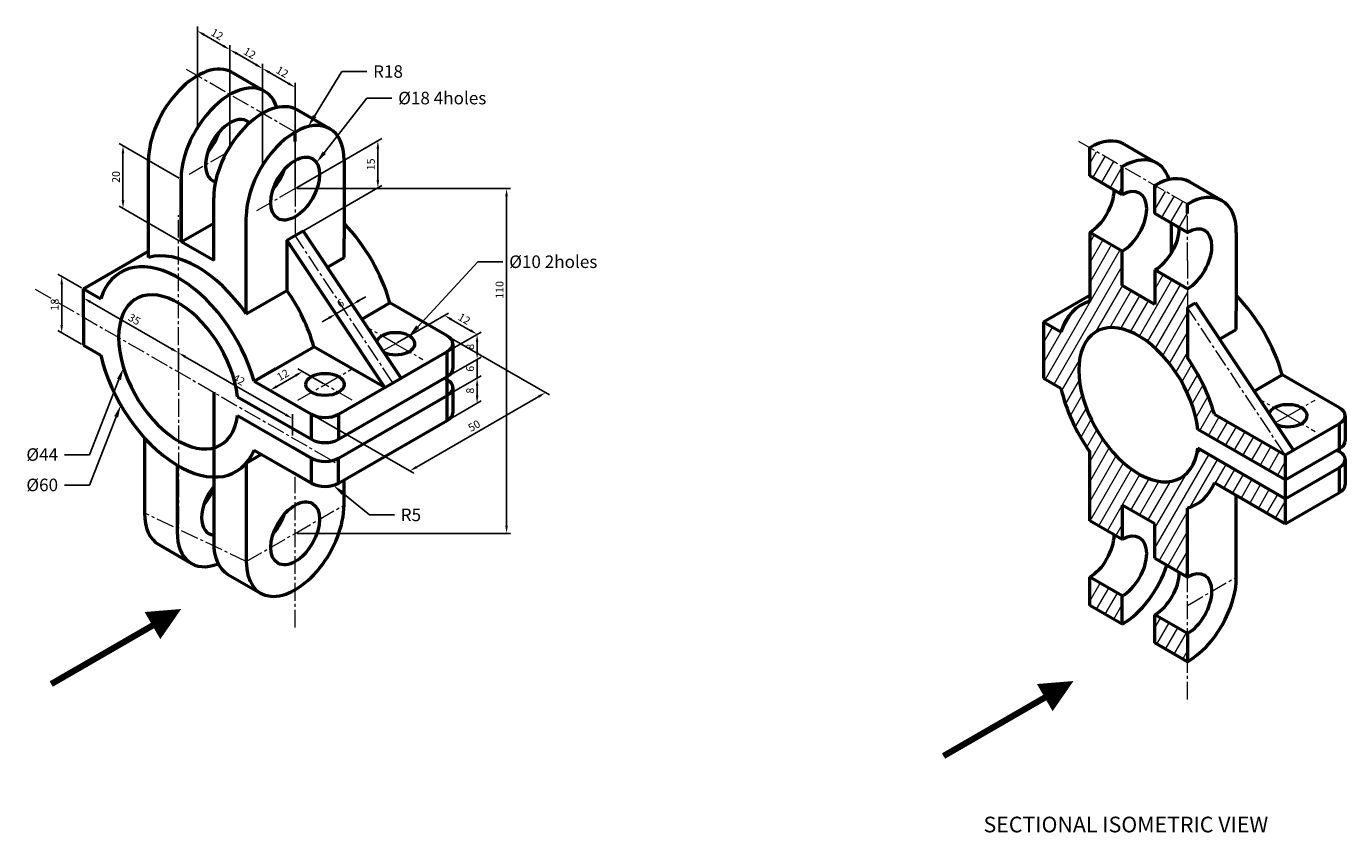
# Model space of a CAD drawing. Units: millimetres. Extents: x 2364 to 2785, y 1000 to 1694.
# Tile 2 of 2: x 2364 to 2785, y 1437 to 1694. Entities that reach past the tile are written whole.
import ezdxf
from ezdxf import colors
from ezdxf.entities.mleader import LeaderData, LeaderLine
from ezdxf.math import Vec2, Vec3

# ---------------------------------------------------------------- set-up
doc = ezdxf.new("R2010")
doc.units = ezdxf.units.MM
doc.linetypes.add('CENTER2', pattern=[28.575, 19.05, -3.175, 3.175, -3.175])
for name, color, linetype, lineweight in [('M-CNTR', 1, 'CENTER2', 18), ('M-DIMS', 2, 'Continuous', 25), ('M-HATC', 8, 'Continuous', 18), ('M-OUTL', 7, 'Continuous', 50), ('M-SYMB', 7, 'Continuous', 18), ('M-TEXT', 3, 'Continuous', 25)]:
    doc.layers.add(name, color=color, linetype=linetype, lineweight=lineweight)
doc.styles.get("Standard").update_dxf_attribs({"font": 'arial.ttf'})
doc.dimstyles.new('ISO-25', dxfattribs={"dimtxt": 2.5, "dimasz": 2.5, "dimexe": 1.25, "dimexo": 0.625, "dimtad": 1, "dimtxsty": 'Standard', "dimcen": 2.5, "dimadec": 0, "dimazin": 0, "dimtfac": 1, "dimtmove": 0, "dimatfit": 3, "dimfxl": 1, "dimarcsym": 0})
pattern_1 = [(60, (-235.2593, 567.1468), (-2.7496307, 1.5875), [])]

# ---------------------------------------------------------------- blocks, each defined once
blk = doc.blocks.new('*D1')
at = {"layer": 'Defpoints', "color": 0, "transparency": 16777216}
for p in [(2439.77, 1680.8), (2439.77, 1648.49), (2450.16, 1642.49)]:
    blk.add_point(p, dxfattribs=at)
at = {"layer": 'M-DIMS', "color": 0, "lineweight": -2, "transparency": 16777216}
for p, q in [((2439.77, 1649.21), (2439.77, 1682.25)), ((2448, 1676.05), (2441.94, 1679.55)), ((2450.16, 1643.21), (2450.16, 1676.25))]:
    blk.add_line(p, q, dxfattribs=at)
at = {"layer": 'M-DIMS', "color": 0, "transparency": 16777216}
for points in [[(2442.15, 1679.91), (2441.73, 1679.19), (2439.77, 1680.8)], [(2448.21, 1676.41), (2447.79, 1675.69), (2450.16, 1674.8)]]:
    blk.add_solid(points, dxfattribs=at)
at = {"layer": 'M-DIMS', "color": 0, "transparency": 16777216, "insert": (2445.91, 1679.43), "char_height": 2.5, "attachment_point": 5, "rotation": 330}
blk.add_mtext('12', dxfattribs=at)
blk = doc.blocks.new('*D2')
at = {"layer": 'Defpoints', "color": 0, "transparency": 16777216}
for p in [(2429.38, 1686.8), (2429.38, 1654.49), (2439.77, 1648.49)]:
    blk.add_point(p, dxfattribs=at)
at = {"layer": 'M-DIMS', "color": 0, "lineweight": -2, "transparency": 16777216}
for p, q in [((2429.38, 1655.21), (2429.38, 1688.25)), ((2437.61, 1682.05), (2431.55, 1685.55)), ((2439.77, 1649.21), (2439.77, 1682.25))]:
    blk.add_line(p, q, dxfattribs=at)
at = {"layer": 'M-DIMS', "color": 0, "transparency": 16777216}
for points in [[(2431.75, 1685.91), (2431.34, 1685.19), (2429.38, 1686.8)], [(2437.82, 1682.41), (2437.4, 1681.69), (2439.77, 1680.8)]]:
    blk.add_solid(points, dxfattribs=at)
at = {"layer": 'M-DIMS', "color": 0, "transparency": 16777216, "insert": (2435.52, 1685.43), "char_height": 2.5, "attachment_point": 5, "rotation": 330}
blk.add_mtext('12', dxfattribs=at)
blk = doc.blocks.new('*D3')
at = {"layer": 'Defpoints', "color": 0, "transparency": 16777216}
for p in [(2418.99, 1692.8), (2418.99, 1660.49), (2429.38, 1654.49)]:
    blk.add_point(p, dxfattribs=at)
at = {"layer": 'M-DIMS', "color": 0, "lineweight": -2, "transparency": 16777216}
for p, q in [((2418.99, 1661.21), (2418.99, 1694.25)), ((2427.22, 1688.05), (2421.15, 1691.55)), ((2429.38, 1655.21), (2429.38, 1688.25))]:
    blk.add_line(p, q, dxfattribs=at)
at = {"layer": 'M-DIMS', "color": 0, "transparency": 16777216}
for points in [[(2421.36, 1691.91), (2420.94, 1691.19), (2418.99, 1692.8)], [(2427.42, 1688.41), (2427.01, 1687.69), (2429.38, 1686.8)]]:
    blk.add_solid(points, dxfattribs=at)
at = {"layer": 'M-DIMS', "color": 0, "transparency": 16777216, "insert": (2425.12, 1691.43), "char_height": 2.5, "attachment_point": 5, "rotation": 330}
blk.add_mtext('12', dxfattribs=at)
blk = doc.blocks.new('*D4')
at = {"layer": 'Defpoints', "color": 0, "transparency": 16777216}
for p in [(2413.79, 1645.49), (2395.26, 1636.19), (2413.79, 1625.49)]:
    blk.add_point(p, dxfattribs=at)
at = {"layer": 'M-DIMS', "color": 0, "lineweight": -2, "transparency": 16777216}
for p, q in [((2413.17, 1645.85), (2394.01, 1656.91)), ((2395.26, 1653.69), (2395.26, 1638.69)), ((2413.17, 1625.85), (2394.01, 1636.91))]:
    blk.add_line(p, q, dxfattribs=at)
at = {"layer": 'M-DIMS', "color": 0, "transparency": 16777216}
for points in [[(2394.84, 1653.69), (2395.68, 1653.69), (2395.26, 1656.19)], [(2394.84, 1638.69), (2395.68, 1638.69), (2395.26, 1636.19)]]:
    blk.add_solid(points, dxfattribs=at)
at = {"layer": 'M-DIMS', "color": 0, "transparency": 16777216, "insert": (2393.36, 1646.19), "char_height": 2.5, "attachment_point": 5, "rotation": 90}
blk.add_mtext('20', dxfattribs=at)
blk = doc.blocks.new('*D5')
at = {"layer": 'Defpoints', "color": 0, "transparency": 16777216}
for p in [(2450.16, 1642.49), (2476.54, 1642.72), (2450.16, 1627.49)]:
    blk.add_point(p, dxfattribs=at)
at = {"layer": 'M-DIMS', "color": 0, "lineweight": -2, "transparency": 16777216}
for p, q in [((2450.79, 1642.85), (2477.79, 1658.44)), ((2476.54, 1655.22), (2476.54, 1645.22)), ((2450.79, 1627.85), (2477.79, 1643.44))]:
    blk.add_line(p, q, dxfattribs=at)
at = {"layer": 'M-DIMS', "color": 0, "transparency": 16777216}
for points in [[(2476.13, 1655.22), (2476.96, 1655.22), (2476.54, 1657.72)], [(2476.13, 1645.22), (2476.96, 1645.22), (2476.54, 1642.72)]]:
    blk.add_solid(points, dxfattribs=at)
at = {"layer": 'M-DIMS', "color": 0, "transparency": 16777216, "insert": (2474.64, 1650.22), "char_height": 2.5, "attachment_point": 5, "rotation": 90}
blk.add_mtext('15', dxfattribs=at)
blk = doc.blocks.new('*D6')
at = {"layer": 'Defpoints', "color": 0, "transparency": 16777216}
for p in [(2442.14, 1578.13), (2459.69, 1579.99), (2449.3, 1573.99)]:
    blk.add_point(p, dxfattribs=at)
at = {"layer": 'M-DIMS', "color": 0, "lineweight": -2, "transparency": 16777216}
for p, q in [((2450.37, 1582.88), (2444.31, 1579.38)), ((2459.07, 1580.35), (2451.28, 1584.85)), ((2448.67, 1574.35), (2440.89, 1578.85))]:
    blk.add_line(p, q, dxfattribs=at)
at = {"layer": 'M-DIMS', "color": 0, "transparency": 16777216}
for points in [[(2450.16, 1583.24), (2450.58, 1582.51), (2452.53, 1584.13)], [(2444.1, 1579.74), (2444.51, 1579.01), (2442.14, 1578.13)]]:
    blk.add_solid(points, dxfattribs=at)
at = {"layer": 'M-DIMS', "color": 0, "transparency": 16777216, "insert": (2446.4, 1582.75), "char_height": 2.5, "attachment_point": 5, "rotation": 30}
blk.add_mtext('12', dxfattribs=at)
blk = doc.blocks.new('*D7')
at = {"layer": 'Defpoints', "color": 0, "transparency": 16777216}
for p in [(2508.2, 1596), (2482.21, 1592.99), (2492.6, 1586.99)]:
    blk.add_point(p, dxfattribs=at)
at = {"layer": 'M-DIMS', "color": 0, "lineweight": -2, "transparency": 16777216}
for p, q in [((2482.83, 1593.35), (2499.06, 1602.72)), ((2499.98, 1600.75), (2506.04, 1597.25)), ((2493.22, 1587.35), (2509.45, 1596.72))]:
    blk.add_line(p, q, dxfattribs=at)
at = {"layer": 'M-DIMS', "color": 0, "transparency": 16777216}
for points in [[(2500.19, 1601.11), (2499.77, 1600.39), (2497.81, 1602)], [(2506.25, 1597.61), (2505.83, 1596.89), (2508.2, 1596)]]:
    blk.add_solid(points, dxfattribs=at)
at = {"layer": 'M-DIMS', "color": 0, "transparency": 16777216, "insert": (2503.95, 1600.63), "char_height": 2.5, "attachment_point": 5, "rotation": 330}
blk.add_mtext('12', dxfattribs=at)
blk = doc.blocks.new('*D8')
at = {"layer": 'Defpoints', "color": 0, "transparency": 16777216}
for p in [(2498.66, 1576.49), (2508.2, 1574), (2498.66, 1568.49)]:
    blk.add_point(p, dxfattribs=at)
at = {"layer": 'M-DIMS', "color": 0, "lineweight": -2, "transparency": 16777216}
for p, q in [((2499.29, 1576.85), (2509.45, 1582.72)), ((2508.2, 1579.5), (2508.2, 1576.5)), ((2499.29, 1568.85), (2509.45, 1574.72))]:
    blk.add_line(p, q, dxfattribs=at)
at = {"layer": 'M-DIMS', "color": 0, "transparency": 16777216}
for points in [[(2507.79, 1579.5), (2508.62, 1579.5), (2508.2, 1582)], [(2507.79, 1576.5), (2508.62, 1576.5), (2508.2, 1574)]]:
    blk.add_solid(points, dxfattribs=at)
at = {"layer": 'M-DIMS', "color": 0, "transparency": 16777216, "insert": (2506.3, 1578), "char_height": 2.5, "attachment_point": 5, "rotation": 90}
blk.add_mtext('8', dxfattribs=at)
blk = doc.blocks.new('*D9')
at = {"layer": 'Defpoints', "color": 0, "transparency": 16777216}
for p in [(2508.2, 1588), (2498.66, 1582.49), (2498.66, 1576.49)]:
    blk.add_point(p, dxfattribs=at)
at = {"layer": 'M-DIMS', "color": 0, "lineweight": -2, "transparency": 16777216}
for p, q in [((2508.2, 1590.5), (2508.2, 1593)), ((2499.29, 1582.85), (2509.45, 1588.72)), ((2508.2, 1582), (2508.2, 1588)), ((2499.29, 1576.85), (2509.45, 1582.72)), ((2508.2, 1579.5), (2508.2, 1577))]:
    blk.add_line(p, q, dxfattribs=at)
at = {"layer": 'M-DIMS', "color": 0, "transparency": 16777216}
for points in [[(2507.79, 1590.5), (2508.62, 1590.5), (2508.2, 1588)], [(2507.79, 1579.5), (2508.62, 1579.5), (2508.2, 1582)]]:
    blk.add_solid(points, dxfattribs=at)
at = {"layer": 'M-DIMS', "color": 0, "transparency": 16777216, "insert": (2506.3, 1585), "char_height": 2.5, "attachment_point": 5, "rotation": 90}
blk.add_mtext('6', dxfattribs=at)
blk = doc.blocks.new('*D10')
at = {"layer": 'Defpoints', "color": 0, "transparency": 16777216}
for p in [(2508.2, 1596), (2498.66, 1590.49), (2498.66, 1582.49)]:
    blk.add_point(p, dxfattribs=at)
at = {"layer": 'M-DIMS', "color": 0, "lineweight": -2, "transparency": 16777216}
for p, q in [((2499.29, 1590.85), (2509.45, 1596.72)), ((2508.2, 1590.5), (2508.2, 1593.5)), ((2499.29, 1582.85), (2509.45, 1588.72))]:
    blk.add_line(p, q, dxfattribs=at)
at = {"layer": 'M-DIMS', "color": 0, "transparency": 16777216}
for points in [[(2507.79, 1593.5), (2508.62, 1593.5), (2508.2, 1596)], [(2507.79, 1590.5), (2508.62, 1590.5), (2508.2, 1588)]]:
    blk.add_solid(points, dxfattribs=at)
at = {"layer": 'M-DIMS', "color": 0, "transparency": 16777216, "insert": (2506.3, 1592), "char_height": 2.5, "attachment_point": 5, "rotation": 90}
blk.add_mtext('8', dxfattribs=at)
blk = doc.blocks.new('*D11')
at = {"layer": 'Defpoints', "color": 0, "transparency": 16777216}
for p in [(2450.16, 1642.49), (2517.59, 1642.49), (2450.16, 1532.49)]:
    blk.add_point(p, dxfattribs=at)
at = {"layer": 'M-DIMS', "color": 0, "lineweight": -2, "transparency": 16777216}
for p, q in [((2450.79, 1642.49), (2518.84, 1642.49)), ((2517.59, 1534.99), (2517.59, 1639.99)), ((2450.79, 1532.49), (2518.84, 1532.49))]:
    blk.add_line(p, q, dxfattribs=at)
at = {"layer": 'M-DIMS', "color": 0, "transparency": 16777216}
for points in [[(2517.17, 1639.99), (2518, 1639.99), (2517.59, 1642.49)], [(2517.17, 1534.99), (2518, 1534.99), (2517.59, 1532.49)]]:
    blk.add_solid(points, dxfattribs=at)
at = {"layer": 'M-DIMS', "color": 0, "transparency": 16777216, "insert": (2515.68, 1610.16), "char_height": 2.5, "attachment_point": 5, "rotation": 90}
blk.add_mtext('110', dxfattribs=at)
blk = doc.blocks.new('*D12')
at = {"layer": 'Defpoints', "color": 0, "transparency": 16777216}
for p in [(2498.66, 1595.49), (2530.02, 1577.39), (2455.36, 1570.49)]:
    blk.add_point(p, dxfattribs=at)
at = {"layer": 'M-DIMS', "color": 0, "lineweight": -2, "transparency": 16777216}
for p, q in [((2499.29, 1595.13), (2531.27, 1576.67)), ((2488.88, 1553.64), (2527.85, 1576.14)), ((2455.99, 1570.13), (2487.97, 1551.67))]:
    blk.add_line(p, q, dxfattribs=at)
at = {"layer": 'M-DIMS', "color": 0, "transparency": 16777216}
for points in [[(2527.64, 1576.5), (2528.06, 1575.78), (2530.02, 1577.39)], [(2488.67, 1554), (2489.09, 1553.28), (2486.72, 1552.39)]]:
    blk.add_solid(points, dxfattribs=at)
at = {"layer": 'M-DIMS', "color": 0, "transparency": 16777216, "insert": (2507.42, 1566.54), "char_height": 2.5, "attachment_point": 5, "rotation": 30}
blk.add_mtext('50', dxfattribs=at)
blk = doc.blocks.new('*D13')
at = {"layer": 'Defpoints', "color": 0, "transparency": 16777216}
for p in [(2468.35, 1605.49), (2468.35, 1605.49), (2463.16, 1602.49)]:
    blk.add_point(p, dxfattribs=at)
at = {"layer": 'M-DIMS', "color": 0, "lineweight": -2, "transparency": 16777216}
for p, q in [((2470.52, 1606.74), (2472.68, 1607.99)), ((2462.84, 1603.03), (2462.53, 1603.58)), ((2463.16, 1602.49), (2468.35, 1605.49)), ((2468.04, 1606.03), (2467.73, 1606.58)), ((2460.99, 1601.24), (2458.82, 1599.99))]:
    blk.add_line(p, q, dxfattribs=at)
at = {"layer": 'M-DIMS', "color": 0, "transparency": 16777216}
for points in [[(2470.31, 1607.1), (2470.72, 1606.38), (2468.35, 1605.49)], [(2460.78, 1601.6), (2461.2, 1600.88), (2463.16, 1602.49)]]:
    blk.add_solid(points, dxfattribs=at)
at = {"layer": 'M-DIMS', "color": 0, "transparency": 16777216, "insert": (2464.8, 1605.64), "char_height": 2.5, "attachment_point": 5, "rotation": 30}
blk.add_mtext('6', dxfattribs=at)
blk = doc.blocks.new('*D14')
at = {"layer": 'Defpoints', "color": 0, "transparency": 16777216}
for p in [(2412.93, 1583.99), (2449.3, 1569.11), (2449.3, 1562.99)]:
    blk.add_point(p, dxfattribs=at)
at = {"layer": 'M-DIMS', "color": 0, "lineweight": -2, "transparency": 16777216}
for p, q in [((2412.93, 1584.71), (2412.93, 1591.55)), ((2415.09, 1588.86), (2447.13, 1570.36)), ((2449.3, 1563.71), (2449.3, 1570.55))]:
    blk.add_line(p, q, dxfattribs=at)
at = {"layer": 'M-DIMS', "color": 0, "transparency": 16777216}
for points in [[(2415.3, 1589.22), (2414.88, 1588.5), (2412.93, 1590.11)], [(2447.34, 1570.72), (2446.93, 1570), (2449.3, 1569.11)]]:
    blk.add_solid(points, dxfattribs=at)
at = {"layer": 'M-DIMS', "color": 0, "transparency": 16777216, "insert": (2432.05, 1581.23), "char_height": 2.5, "attachment_point": 5, "rotation": 330}
blk.add_mtext('42', dxfattribs=at)
blk = doc.blocks.new('*D15')
at = {"layer": 'Defpoints', "color": 0, "transparency": 16777216}
for p in [(2382.61, 1610.49), (2375.71, 1596.48), (2382.61, 1592.49)]:
    blk.add_point(p, dxfattribs=at)
at = {"layer": 'M-DIMS', "color": 0, "lineweight": -2, "transparency": 16777216}
for p, q in [((2381.99, 1610.85), (2374.46, 1615.2)), ((2375.71, 1611.98), (2375.71, 1598.98)), ((2381.99, 1592.85), (2374.46, 1597.2))]:
    blk.add_line(p, q, dxfattribs=at)
at = {"layer": 'M-DIMS', "color": 0, "transparency": 16777216}
for points in [[(2375.3, 1611.98), (2376.13, 1611.98), (2375.71, 1614.48)], [(2375.3, 1598.98), (2376.13, 1598.98), (2375.71, 1596.48)]]:
    blk.add_solid(points, dxfattribs=at)
at = {"layer": 'M-DIMS', "color": 0, "transparency": 16777216, "insert": (2373.81, 1605.48), "char_height": 2.5, "attachment_point": 5, "rotation": 90}
blk.add_mtext('18', dxfattribs=at)
blk = doc.blocks.new('*D16')
at = {"layer": 'Defpoints', "color": 0, "transparency": 16777216}
for p in [(2382.61, 1607.61), (2382.61, 1601.49), (2412.93, 1583.99)]:
    blk.add_point(p, dxfattribs=at)
at = {"layer": 'M-DIMS', "color": 0, "lineweight": -2, "transparency": 16777216}
for p, q in [((2382.61, 1602.21), (2382.61, 1609.05)), ((2410.76, 1591.36), (2384.78, 1606.36)), ((2412.93, 1584.71), (2412.93, 1591.55))]:
    blk.add_line(p, q, dxfattribs=at)
at = {"layer": 'M-DIMS', "color": 0, "transparency": 16777216}
for points in [[(2384.99, 1606.72), (2384.57, 1606), (2382.61, 1607.61)], [(2410.97, 1591.72), (2410.55, 1591), (2412.93, 1590.11)]]:
    blk.add_solid(points, dxfattribs=at)
at = {"layer": 'M-DIMS', "color": 0, "transparency": 16777216, "insert": (2398.72, 1600.5), "char_height": 2.5, "attachment_point": 5, "rotation": 330}
blk.add_mtext('35', dxfattribs=at)

msp = doc.modelspace()

# ---------------------------------------------------------------- hatches: boundary and pattern name
at = {"layer": 'M-HATC'}
h = msp.add_hatch(dxfattribs=at)
h.set_pattern_fill('ANSI31', color=256, angle=15)
h.set_pattern_definition(pattern_1)
h.paths.add_polyline_path([(2713.969, 1640.521), (2713.969, 1649.521), (2703.577, 1655.521), (2703.577, 1646.521)])
h.paths.add_polyline_path([(2724.361, 1643.521), (2724.361, 1634.521), (2734.754, 1628.521), (2734.754, 1634.521), (2734.754, 1637.521)])
h = msp.add_hatch(dxfattribs=at)
h.set_pattern_fill('ANSI31', color=256, angle=15)
h.set_pattern_definition(pattern_1)
edge = h.paths.add_edge_path()
edge.add_line((2724.361, 1535.521), (2724.361, 1524.521))
edge.add_line((2724.361, 1524.521), (2734.754, 1518.521))
edge.add_line((2734.754, 1518.521), (2734.754, 1540.521))
edge.add_ellipse((2719.165, 1573.521), major_axis=(18.371, -31.82), ratio=0.5773503, start_angle=355.285, end_angle=374.08568)
edge.add_line((2743.336, 1548.566), (2765.931, 1535.521))
edge.add_line((2765.931, 1535.521), (2765.931, 1543.521))
edge.add_line((2765.931, 1543.521), (2738.04, 1559.624))
edge.add_ellipse((2719.165, 1573.521), major_axis=(13.472, -23.335), ratio=0.5773503, start_angle=37.29525, end_angle=383.636, ccw=False)
edge.add_line((2738.04, 1565.624), (2765.931, 1549.521))
edge.add_line((2765.931, 1549.521), (2765.931, 1557.521))
edge.add_line((2765.931, 1557.521), (2743.336, 1570.566))
edge.add_ellipse((2719.165, 1573.521), major_axis=(18.371, -31.82), ratio=0.5773503, start_angle=53.02936, end_angle=103.89789)
edge.add_line((2734.754, 1588.521), (2734.754, 1604.521))
edge.add_line((2734.754, 1604.521), (2734.754, 1610.521))
edge.add_line((2734.754, 1610.521), (2724.361, 1616.521))
edge.add_line((2724.361, 1616.521), (2724.361, 1605.521))
edge.add_line((2724.361, 1605.521), (2713.969, 1611.521))
edge.add_line((2713.969, 1611.521), (2713.969, 1622.521))
edge.add_line((2713.969, 1622.521), (2703.577, 1628.521))
edge.add_line((2703.577, 1628.521), (2703.577, 1606.521))
edge.add_ellipse((2719.165, 1573.521), major_axis=(18.371, -31.82), ratio=0.5773503, start_angle=175.285, end_angle=196.75667)
edge.add_line((2694.381, 1596.83), (2688.854, 1600.021))
edge.add_line((2688.854, 1600.021), (2688.854, 1582.021))
edge.add_line((2688.854, 1582.021), (2694.381, 1578.83))
edge.add_ellipse((2719.165, 1573.521), major_axis=(18.371, -31.82), ratio=0.5773503, start_angle=227.90919, end_angle=283.89789)
edge.add_line((2703.577, 1558.521), (2703.577, 1536.521))
edge.add_line((2703.577, 1536.521), (2713.969, 1530.521))
edge.add_line((2713.969, 1530.521), (2713.969, 1541.521))
edge.add_line((2713.969, 1541.521), (2724.361, 1535.521))
h = msp.add_hatch(dxfattribs=at)
h.set_pattern_fill('ANSI31', color=256, angle=15)
h.set_pattern_definition(pattern_1)
h.paths.add_polyline_path([(2703.577, 1518.521), (2703.577, 1509.521), (2713.969, 1503.521), (2713.969, 1512.521)])
h.paths.add_polyline_path([(2734.754, 1491.521), (2734.754, 1500.521), (2724.361, 1506.521), (2724.361, 1497.521)])

# ---------------------------------------------------------------- linework, layer by layer
at = {"layer": 'M-CNTR', "ltscale": 0.3}
for p, q in [((2450.165, 1660.493), (2415.452, 1680.535)), ((2429.38, 1655.91), (2429.38, 1669.493)), ((2428.153, 1653.785), (2416.39, 1646.993)), ((2450.165, 1642.493), (2450.165, 1657.493)), ((2734.754, 1637.521), (2700.04, 1657.563)), ((2450.165, 1642.493), (2463.155, 1649.993)), ((2450.165, 1642.493), (2437.174, 1634.993)), ((2450.165, 1642.493), (2450.165, 1627.493)), ((2412.926, 1583.993), (2412.926, 1633.993)), ((2734.754, 1619.521), (2734.754, 1634.521)), ((2481.342, 1580.493), (2450.165, 1627.493)), ((2734.754, 1619.521), (2734.754, 1604.521)), ((2367.247, 1610.366), (2464.021, 1554.493)), ((2765.931, 1557.521), (2734.754, 1604.521)), ((2482.208, 1592.993), (2473.547, 1597.993)), ((2482.208, 1592.993), (2490.868, 1597.993)), ((2482.208, 1592.993), (2490.868, 1587.993)), ((2412.926, 1583.993), (2412.926, 1533.993)), ((2766.797, 1570.021), (2758.136, 1575.021)), ((2766.797, 1570.021), (2775.457, 1575.021)), ((2766.797, 1570.021), (2775.457, 1565.021)), ((2450.165, 1502.399), (2450.165, 1550.488)), ((2450.165, 1532.493), (2465.753, 1541.493)), ((2434.576, 1523.493), (2402.137, 1538.975)), ((2434.576, 1523.493), (2450.165, 1532.493)), ((2734.754, 1509.521), (2750.342, 1518.521)), ((2734.754, 1479.427), (2734.754, 1518.521))]:
    msp.add_line(p, q, dxfattribs=at)
at = {"layer": 'M-CNTR'}
for p, q in [((2482.208, 1592.993), (2478.184, 1590.67)), ((2766.797, 1570.021), (2762.773, 1567.698))]:
    msp.add_line(p, q, dxfattribs=at)
at = {"layer": 'M-CNTR', "ltscale": 0.3}
for points in [[(2468.351, 1574.993), (2459.691, 1579.993), (2451.031, 1584.993)], [(2451.031, 1574.993), (2459.691, 1579.993), (2468.351, 1584.993)]]:
    msp.add_lwpolyline(points, dxfattribs=at)
at = {"layer": 'M-OUTL'}
for p, q in [((2430.01, 1679.585), (2440.403, 1673.585)), ((2461.187, 1661.585), (2450.795, 1667.585)), ((2450.165, 1657.493), (2450.165, 1660.493)), ((2703.577, 1646.521), (2703.577, 1655.521)), ((2714.599, 1656.613), (2724.992, 1650.613)), ((2403.399, 1620.493), (2403.399, 1651.493)), ((2465.753, 1651.493), (2465.753, 1626.493)), ((2713.969, 1640.521), (2713.969, 1649.521)), ((2413.792, 1625.493), (2413.792, 1645.493)), ((2413.792, 1645.493), (2413.792, 1625.493)), ((2713.969, 1640.521), (2703.577, 1646.521)), ((2724.361, 1634.521), (2724.361, 1643.521)), ((2745.776, 1638.613), (2735.384, 1644.613)), ((2424.184, 1619.493), (2424.184, 1639.493)), ((2734.754, 1634.521), (2734.754, 1637.521)), ((2434.576, 1602.493), (2434.576, 1633.493)), ((2734.754, 1628.521), (2724.361, 1634.521)), ((2413.792, 1625.493), (2424.184, 1631.493)), ((2447.567, 1625.993), (2452.763, 1628.993)), ((2483.94, 1581.993), (2452.763, 1628.993)), ((2713.969, 1622.521), (2703.577, 1628.521)), ((2703.577, 1628.521), (2703.577, 1606.521)), ((2729.557, 1631.521), (2729.557, 1621.813)), ((2750.342, 1628.521), (2750.342, 1603.521)), ((2424.184, 1619.493), (2413.792, 1625.493)), ((2478.744, 1578.993), (2447.567, 1625.993)), ((2447.567, 1625.993), (2447.567, 1609.993)), ((2465.753, 1620.493), (2465.753, 1626.493)), ((2382.615, 1610.493), (2403.399, 1622.493)), ((2460.437, 1617.424), (2465.753, 1620.493)), ((2713.969, 1611.521), (2713.969, 1622.521)), ((2734.754, 1610.521), (2724.361, 1616.521)), ((2724.361, 1616.521), (2724.361, 1605.521)), ((2724.361, 1605.521), (2713.969, 1611.521)), ((2382.615, 1601.493), (2382.615, 1610.493)), ((2382.615, 1610.493), (2388.142, 1607.302)), ((2434.576, 1602.493), (2447.567, 1609.993)), ((2688.854, 1600.021), (2703.577, 1608.521)), ((2471.426, 1600.858), (2480.398, 1606.038)), ((2498.662, 1595.493), (2480.398, 1606.038)), ((2734.754, 1604.521), (2737.352, 1606.021)), ((2734.754, 1604.521), (2734.754, 1588.521)), ((2768.529, 1559.021), (2737.352, 1606.021)), ((2750.342, 1597.521), (2750.342, 1603.521)), ((2382.615, 1601.493), (2382.615, 1592.493)), ((2688.854, 1600.021), (2694.381, 1596.83)), ((2688.854, 1600.021), (2688.854, 1582.021)), ((2745.026, 1594.452), (2750.342, 1597.521)), ((2382.615, 1592.493), (2388.142, 1589.302)), ((2437.097, 1581.038), (2456.149, 1592.038)), ((2478.744, 1578.993), (2456.149, 1592.038)), ((2464.021, 1570.493), (2498.662, 1590.493)), ((2498.662, 1568.493), (2498.662, 1590.493)), ((2500.456, 1592.993), (2500.456, 1584.993)), ((2437.097, 1581.038), (2444.025, 1585.038)), ((2464.021, 1562.493), (2498.662, 1582.493)), ((2688.854, 1582.021), (2694.381, 1578.83)), ((2756.015, 1577.886), (2764.987, 1583.066)), ((2783.251, 1572.521), (2764.987, 1583.066)), ((2437.097, 1581.038), (2455.361, 1570.493)), ((2478.744, 1578.993), (2483.94, 1581.993)), ((2500.456, 1578.993), (2500.456, 1570.993)), ((2424.184, 1577.493), (2424.184, 1529.493)), ((2431.8, 1576.096), (2455.361, 1562.493)), ((2464.021, 1556.493), (2498.662, 1576.493)), ((2431.8, 1570.096), (2449.299, 1559.993)), ((2455.361, 1562.493), (2455.361, 1570.493)), ((2464.021, 1570.493), (2464.021, 1562.493)), ((2743.336, 1570.566), (2765.931, 1557.521)), ((2785.045, 1570.021), (2785.045, 1562.021)), ((2464.021, 1548.493), (2498.662, 1568.493)), ((2765.931, 1549.521), (2738.04, 1565.624)), ((2765.931, 1557.521), (2783.251, 1567.521)), ((2783.251, 1558.521), (2783.251, 1567.521)), ((2402.137, 1562.931), (2402.137, 1538.975)), ((2434.576, 1554.91), (2439.411, 1557.702)), ((2437.097, 1559.038), (2449.299, 1551.993)), ((2449.299, 1559.993), (2455.361, 1556.493)), ((2703.577, 1536.521), (2703.577, 1558.521)), ((2765.931, 1543.521), (2738.04, 1559.624)), ((2765.931, 1549.521), (2783.251, 1559.521)), ((2765.931, 1557.521), (2768.529, 1559.021)), ((2765.931, 1557.521), (2765.931, 1535.521)), ((2412.529, 1554.226), (2412.529, 1532.975)), ((2434.576, 1554.91), (2434.576, 1523.493)), ((2455.361, 1548.493), (2455.361, 1556.493)), ((2464.021, 1548.493), (2464.021, 1556.493)), ((2765.931, 1543.521), (2783.251, 1553.521)), ((2783.251, 1545.521), (2783.251, 1553.521)), ((2785.045, 1556.021), (2785.045, 1548.021)), ((2449.299, 1551.993), (2455.361, 1548.493)), ((2465.753, 1541.493), (2465.753, 1549.493)), ((2765.931, 1535.521), (2743.336, 1548.566)), ((2750.342, 1518.521), (2750.342, 1544.521)), ((2765.931, 1535.521), (2783.251, 1545.521)), ((2724.361, 1535.521), (2713.969, 1541.521)), ((2713.969, 1541.521), (2713.969, 1530.521)), ((2734.754, 1518.521), (2734.754, 1540.521)), ((2713.969, 1530.521), (2703.577, 1536.521)), ((2724.361, 1524.521), (2724.361, 1535.521)), ((2406.702, 1528.884), (2417.095, 1522.884)), ((2724.361, 1524.521), (2734.754, 1518.521)), ((2428.75, 1519.401), (2439.142, 1513.401)), ((2713.969, 1512.521), (2703.577, 1518.521)), ((2703.577, 1509.521), (2703.577, 1518.521)), ((2713.969, 1503.521), (2713.969, 1512.521)), ((2713.969, 1503.521), (2703.577, 1509.521)), ((2734.754, 1500.521), (2724.361, 1506.521)), ((2724.361, 1497.521), (2724.361, 1506.521)), ((2734.754, 1500.521), (2734.754, 1491.521)), ((2734.754, 1491.521), (2724.361, 1497.521))]:
    msp.add_line(p, q, dxfattribs=at)
for centre, major_axis, start_param, end_param in [((2418.988, 1660.493), (-11.023, -19.092), 3.1415927, 5.4977871), ((2429.38, 1654.493), (-11.023, -19.092), 2.65071, 5.4977871), ((2439.772, 1648.493), (-11.023, -19.092), 3.1415927, 5.4977871), ((2429.38, 1654.493), (-5.511, -9.546), 9.276926, 12.7142226), ((2450.165, 1642.493), (-11.023, -19.092), 2.3561945, 5.4977871), ((2418.988, 1660.493), (-5.511, -9.546), 1.2309594, 1.9106332), ((2703.577, 1637.521), (-11.023, -19.092), 3.1415927, 3.9269908), ((2713.969, 1631.521), (-11.023, -19.092), 2.65071, 3.9269908), ((2713.969, 1631.521), (-11.023, -19.092), 2.65071, 3.9269908), ((2439.772, 1648.493), (-5.511, -9.546), 7.5141447, 8.1938185), ((2724.361, 1625.521), (-11.023, -19.092), 3.1415927, 3.9269908), ((2703.577, 1637.521), (-5.511, -9.546), 7.0685835, 8.6393798), ((2713.969, 1631.521), (-5.511, -9.546), 7.0685835, 10.2101761), ((2734.754, 1619.521), (-11.023, -19.092), 2.3561945, 3.9269908), ((2456.227, 1608.993), (18.371, -31.82), 7.4440071, 8.2639562), ((2724.361, 1625.521), (-5.511, -9.546), 7.0685835, 8.6393798), ((2734.754, 1619.521), (-5.511, -9.546), 7.0685835, 10.2101761), ((2412.926, 1583.993), (18.371, -31.82), 7.4440071, 9.9054835), ((2418.988, 1587.493), (18.371, -31.82), 7.9958787, 9.2828809), ((2412.926, 1583.993), (13.472, -23.335), 0.922188, 6.9317936), ((2431.978, 1594.993), (18.371, -31.82), 7.4440071, 7.9958787), ((2740.816, 1586.021), (18.371, -31.82), 7.4440071, 8.2639562), ((2719.165, 1573.521), (18.371, -31.82), 2.9996956, 3.6222982), ((2719.165, 1573.521), (18.371, -31.82), 9.2828809, 9.9054835), ((2719.165, 1573.521), (13.472, -23.335), 0.922188, 6.9317936), ((2482.208, 1592.993), (-6.124, 0), 0.9232054, 6.0914745), ((2494.332, 1592.993), (-6.124, 0), 8.6393798, 10.2101761), ((2412.926, 1583.993), (18.371, -31.82), 4.2316835, 6.6931599), ((2719.165, 1573.521), (18.371, -31.82), 7.4440071, 7.9958787), ((2719.165, 1573.521), (18.371, -31.82), 7.4440071, 7.9958787), ((2719.165, 1573.521), (18.371, -31.82), 1.1608218, 1.7126934), ((2494.332, 1584.993), (-6.124, 0), 2.3561945, 3.1415927), ((2494.332, 1578.993), (-6.124, 0), 2.3561945, 4.1283487), ((2719.165, 1573.521), (18.371, -31.82), 4.2316835, 4.854286), ((2719.165, 1573.521), (18.371, -31.82), 4.2316835, 4.854286), ((2766.797, 1570.021), (-6.124, 0), 0.9232054, 6.0914745), ((2459.691, 1572.993), (-6.124, 0), 0.7853982, 2.3561945), ((2494.332, 1570.993), (-6.124, 0), 2.3561945, 3.1415927), ((2778.921, 1570.021), (-6.124, 0), 8.6393798, 10.2101761), ((2459.691, 1564.993), (-6.124, 0), 0.7853982, 2.3561945), ((2778.921, 1562.021), (-6.124, 0), 2.3561945, 3.1415927), ((2778.921, 1556.021), (-6.124, 0), 2.3561945, 4.1283487), ((2459.691, 1558.993), (-6.124, 0), 7.0685835, 8.6393798), ((2459.691, 1550.993), (-6.124, 0), 0.7853982, 2.3561945), ((2719.165, 1573.521), (18.371, -31.82), 6.1412883, 6.6931599), ((2428.117, 1541.975), (-5.511, -9.546), 4.4559725, 6.5396018), ((2417.725, 1547.975), (-5.511, -9.546), 7.5141447, 8.0453267), ((2778.921, 1548.021), (-6.124, 0), 2.3561945, 3.1415927), ((2450.165, 1532.493), (-11.023, -19.092), 5.4977871, 8.6393798), ((2417.725, 1547.975), (-11.023, -19.092), 5.4977871, 6.2831853), ((2439.772, 1538.493), (-5.511, -9.546), 7.5141447, 8.1938185), ((2428.117, 1541.975), (-11.023, -19.092), 5.4977871, 6.907965), ((2703.577, 1527.521), (-5.511, -9.546), 0.7853982, 2.3561945), ((2713.969, 1521.521), (-5.511, -9.546), 0.7853982, 3.9269908), ((2439.772, 1538.493), (-11.023, -19.092), 5.4977871, 6.2831853), ((2713.969, 1521.521), (-11.023, -19.092), 7.0685835, 8.2153488), ((2724.361, 1515.521), (-5.511, -9.546), 0.7853982, 2.3561945), ((2734.754, 1509.521), (-5.511, -9.546), 0.7853982, 3.9269908), ((2734.754, 1509.521), (-11.023, -19.092), 7.0685835, 8.6393798)]:
    msp.add_ellipse(centre, major_axis=major_axis, ratio=0.5773503, start_param=start_param, end_param=end_param, dxfattribs=at)
for centre, major_axis in [((2450.165, 1642.493), (-5.511, -9.546)), ((2459.691, 1579.993), (-6.124, 0)), ((2450.165, 1532.493), (-5.511, -9.546))]:
    msp.add_ellipse(centre, major_axis=major_axis, ratio=0.5773503, dxfattribs=at)
at = {"layer": 'M-SYMB'}
for points in [[(2404.659, 1503.056, 10, 0, 0), (2413.822, 1508.346, 0, 0, 0)], [(2689.248, 1480.084, 10, 0, 0), (2698.411, 1485.374, 0, 0, 0)]]:
    msp.add_lwpolyline(points, format="xyseb", dxfattribs=at)
at = {"layer": 'M-SYMB', "const_width": 2}
for points in [[(2404.659, 1503.056), (2372.369, 1484.414)], [(2689.248, 1480.084), (2656.958, 1461.441)]]:
    msp.add_lwpolyline(points, dxfattribs=at)

# ---------------------------------------------------------------- texts
at = {"layer": 'M-TEXT', "insert": (2669.707, 1442.09), "char_height": 5, "attachment_point": 1}
msp.add_mtext_dynamic_manual_height_columns('SECTIONAL ISOMETRIC VIEW', width=110.13039, gutter_width=12.5, heights=[0], dxfattribs=at)

# ---------------------------------------------------------------- dimensions: what is measured, and where the dimension line sits
at = {"layer": 'M-DIMS'}
for p1, p2, distance, picture, middle in [((2429.38, 1654.493), (2418.988, 1660.493), -27.98, '*D3', (2425.124, 1691.43)), ((2439.772, 1648.493), (2429.38, 1654.493), -27.98, '*D2', (2435.516, 1685.43)), ((2450.165, 1642.493), (2439.772, 1648.493), -27.98, '*D1', (2445.909, 1679.43)), ((2450.165, 1642.493), (2450.165, 1627.493), 26.377, '*D5', (2474.64, 1650.222)), ((2413.792, 1645.493), (2413.792, 1625.493), -18.531, '*D4', (2393.359, 1646.192)), ((2382.615, 1610.493), (2382.615, 1592.493), -6.902, '*D15', (2373.811, 1605.478)), ((2412.926, 1583.993), (2382.615, 1601.493), -5.294, '*D16', (2398.721, 1600.503)), ((2463.155, 1602.493), (2468.351, 1605.493), 0, '*D13', (2464.802, 1605.64)), ((2482.208, 1592.993), (2492.6, 1586.993), 15.605, '*D7', (2503.949, 1600.631)), ((2455.361, 1570.493), (2498.662, 1595.493), -31.355, '*D12', (2507.415, 1566.537)), ((2498.662, 1582.493), (2498.662, 1590.493), -9.543, '*D10', (2506.303, 1592.003)), ((2412.926, 1583.993), (2449.299, 1562.993), 5.294, '*D14', (2432.052, 1581.234)), ((2498.662, 1576.493), (2498.662, 1582.493), -9.543, '*D9', (2506.303, 1585.003)), ((2459.691, 1579.993), (2449.299, 1573.993), -7.158, '*D6', (2446.397, 1582.754)), ((2498.662, 1576.493), (2498.662, 1568.493), 9.543, '*D8', (2506.303, 1578.003))]:
    dim = msp.add_aligned_dim(p1=p1, p2=p2, distance=distance, dimstyle='ISO-25', override={"dimclrd": 0, "dimclre": 0, "dimclrt": 0}, dxfattribs=at)
    dim.commit()
    dim.dimension.update_dxf_attribs({"geometry": picture, "text_midpoint": middle})
dim = msp.add_linear_dim(base=(2517.586, 1642.493), p1=(2450.165, 1532.493), p2=(2450.165, 1642.493), angle=90, dimstyle='ISO-25', override={"dimclrd": 0, "dimclre": 0, "dimclrt": 0}, dxfattribs=at)
dim.commit()
dim.dimension.update_dxf_attribs({"geometry": '*D11', "text_midpoint": (2517.586, 1610.159), "dimtype": 161})

# ---------------------------------------------------------------- leaders
ml = msp.add_multileader_mtext('Standard', dxfattribs=at)
ml.set_content('R18', color=256)
ml.set_leader_properties()
ml.build(insert=Vec2(0, 0))
ctx = ml.context
ctx.base_point, ctx.plane_origin = Vec3(2473.034, 1679.807), Vec3(2454.298, 1662.235)
notes = []
notes.append((ctx, [(0, (1, 1, 0), (2465.034, 1679.807), (1, 0), 8, [(0, [(2454.298, 1662.235)], 0, [])])]))
ctx.mtext.insert, ctx.mtext.flow_direction = Vec3(2475.034, 1681.841), 5
ml = msp.add_multileader_mtext('Standard', dxfattribs=at)
ml.set_content('%%C18 4holes', color=256)
ml.set_leader_properties()
ml.build(insert=Vec2(0, 0))
ctx = ml.context
ctx.base_point, ctx.plane_origin = Vec3(2481.034, 1671.289), Vec3(2456.978, 1650.797)
notes.append((ctx, [(0, (1, 1, 0), (2473.034, 1671.289), (1, 0), 8, [(0, [(2456.978, 1650.797)], 0, [])])]))
ctx.mtext.insert, ctx.mtext.flow_direction = Vec3(2483.034, 1673.37), 5
ml = msp.add_multileader_mtext('Standard', dxfattribs=at)
ml.set_content('%%C10 2holes', color=256)
ml.set_leader_properties()
ml.build(insert=Vec2(0, 0))
ctx = ml.context
ctx.base_point, ctx.plane_origin = Vec3(2516.442, 1619.071), Vec3(2483.087, 1596.492)
notes.append((ctx, [(0, (1, 1, 0), (2508.442, 1619.071), (1, 0), 8, [(0, [(2486.538, 1595.493)], 0, [])])]))
ctx.mtext.insert, ctx.mtext.flow_direction = Vec3(2518.442, 1621.151), 5
ml = msp.add_multileader_mtext('Standard', dxfattribs=at)
ml.set_content('%%C44', color=256)
ml.set_leader_properties()
ml.build(insert=Vec2(0, 0))
ctx = ml.context
ctx.base_point, ctx.plane_origin = Vec3(2362.49, 1557.546), Vec3(2395.445, 1585.335)
ctx.text_align_type = 2
notes.append((ctx, [(0, (1, 1, 0), (2384.555, 1557.546), (-1, 0), 8, [(0, [(2395.445, 1585.335)], 0, [])])]))
ctx.mtext.insert, ctx.mtext.alignment, ctx.mtext.flow_direction = Vec3(2374.555, 1559.627), 3, 5
ml = msp.add_multileader_mtext('Standard', dxfattribs=at)
ml.set_content('%%C60', color=256)
ml.set_leader_properties()
ml.build(insert=Vec2(0, 0))
ctx = ml.context
ctx.base_point, ctx.plane_origin = Vec3(2362.487, 1547.856), Vec3(2394.554, 1573.387)
ctx.text_align_type = 2
notes.append((ctx, [(0, (1, 1, 0), (2384.555, 1547.856), (-1, 0), 8, [(0, [(2394.554, 1573.387)], 0, [])])]))
ctx.mtext.insert, ctx.mtext.alignment, ctx.mtext.flow_direction = Vec3(2374.555, 1549.937), 3, 5
ml = msp.add_multileader_mtext('Standard', dxfattribs=at)
ml.set_content('R5', color=256)
ml.set_leader_properties()
ml.build(insert=Vec2(0, 0))
ctx = ml.context
ctx.base_point, ctx.plane_origin = Vec3(2481.834, 1538.344), Vec3(2462.335, 1547.804)
notes.append((ctx, [(0, (1, 1, 0), (2473.834, 1538.344), (1, 0), 8, [(0, [(2462.335, 1547.804)], 0, [])])]))
ctx.mtext.insert, ctx.mtext.flow_direction = Vec3(2483.834, 1540.378), 5
for ctx, leaders in notes:
    for number, flags, end, landing, length, lines in leaders:
        leader = LeaderData()
        leader.index, (leader.has_last_leader_line, leader.has_dogleg_vector, leader.attachment_direction) = number, flags
        leader.last_leader_point, leader.dogleg_vector, leader.dogleg_length = Vec3(end), Vec3(landing), length
        for number, points, colour, breaks in lines:
            line = LeaderLine()
            line.index, line.vertices, line.color, line.breaks = number, Vec3.list(points), colors.encode_raw_color(colour), breaks
            leader.lines.append(line)
        ctx.leaders.append(leader)

doc.saveas('drawing.dxf')
